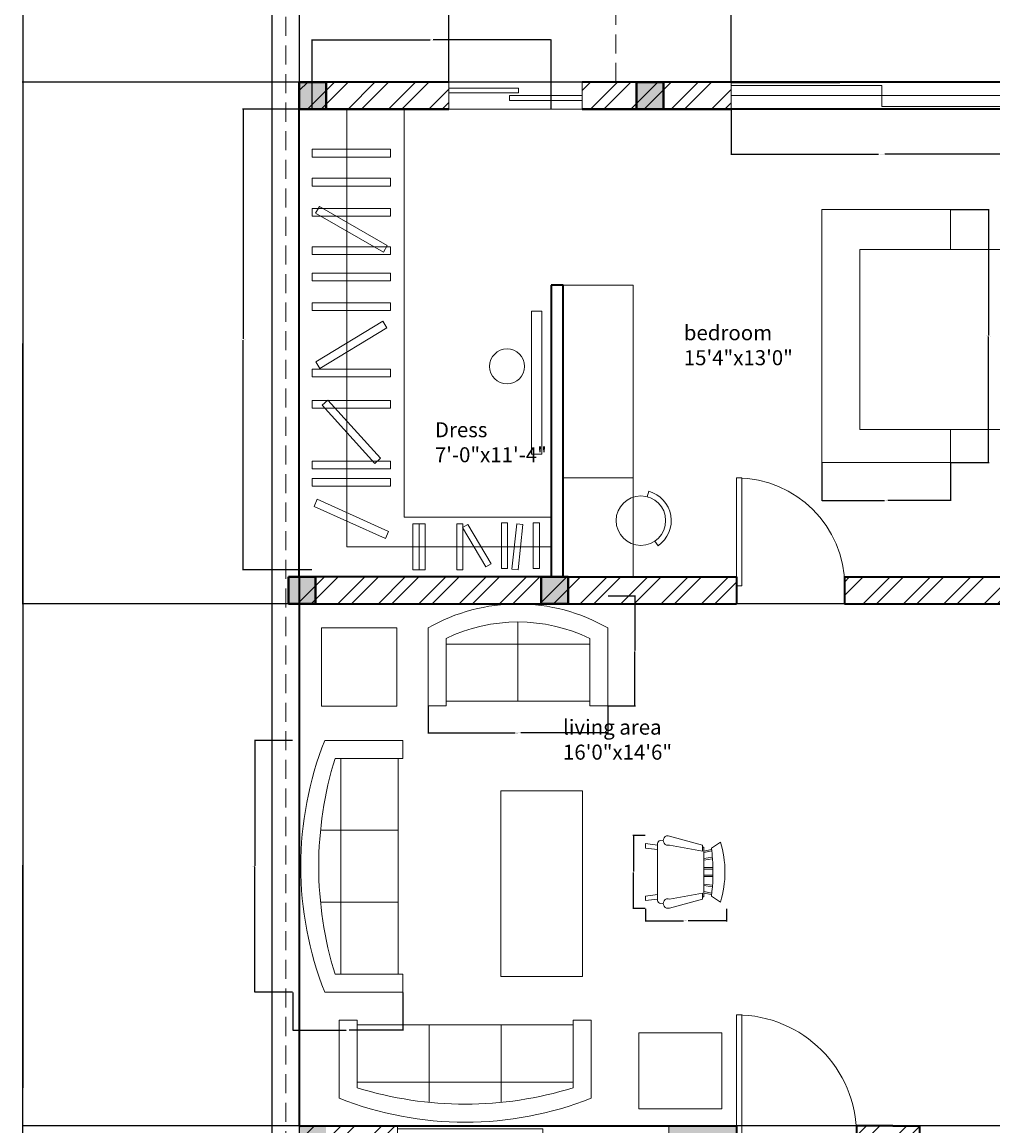
# Model space of a CAD drawing. Units: inches. Extents: x 19613 to 21413, y 12082 to 13202.
# Tile 3 of 9: x 19613 to 19937, y 12634 to 13002. Entities that reach past the tile are written whole.
import ezdxf

# ---------------------------------------------------------------- set-up
doc = ezdxf.new("R2010")
doc.units = ezdxf.units.IN
doc.linetypes.add('HIDDEN', pattern=[9.525, 6.35, -3.175])
for name, color, linetype, lineweight in [('A-ANNO-DIMS', 2, 'Continuous', 18), ('A-AREA-IDEN', 7, 'Continuous', 18), ('A-COLS', 7, 'Continuous', 40), ('A-COLS-PATT', 6, 'Continuous', 13), ('A-DOOR', 3, 'Continuous', 18), ('A-FLOR-CASE', 9, 'Continuous', 18), ('A-FLOR-HIDN', 8, 'HIDDEN', 13), ('A-FURN', 8, 'Continuous', 18), ('A-GLAZ', 4, 'Continuous', 18), ('A-WALL', 7, 'Continuous', 35), ('A-WALL-PATT', 252, 'Continuous', 13), ('C-PROP', 7, 'Continuous', 25), ('C-PROP-HIDN', 8, 'HIDDEN', 13)]:
    doc.layers.add(name, color=color, linetype=linetype, lineweight=lineweight)
doc.styles.get("Standard").update_dxf_attribs({"font": 'arial.ttf'})
doc.dimstyles.get("Standard").update_dxf_attribs({"dimtxt": 0.18, "dimasz": 0.18, "dimexe": 0.18, "dimexo": 0.0625, "dimgap": 0.09, "dimtad": 0, "dimtih": 1, "dimtoh": 1, "dimdec": 4, "dimzin": 0, "dimdsep": 46, "dimtxsty": 'Standard', "dimcen": 0.09, "dimadec": 0, "dimazin": 0, "dimtfac": 1, "dimtdec": 4, "dimtofl": 0, "dimtmove": 0, "dimatfit": 3, "dimfxl": 1, "dimtolj": 1, "dimtzin": 0, "dimarcsym": 0})

# ---------------------------------------------------------------- blocks, each defined once
blk = doc.blocks.new('*U4')
for p, q in [((0, 0), (0, -6)), ((36, 0), (36, -6))]:
    blk.add_line(p, q)
blk.add_lwpolyline([(0, 0), (0, 36), (1.75, 36), (1.75, 0)], close=True)
blk.add_arc((0, 0), 36, 0, 90)
blk = doc.blocks.new('Bed - Queen')
for p, q in [((0, -80.00003), (0, 0)), ((0, 0), (59.99999, 0)), ((59.99999, 0), (59.99999, -80.00003)), ((7.99999, -1.2), (28.79998, -1.2)), ((7.99999, -14.4), (7.99999, -1.2)), ((28.79998, -1.2), (28.79998, -14.4)), ((31.19999, -1.2), (51.99999, -1.2)), ((31.19999, -14.4), (31.19999, -1.2)), ((51.99999, -1.2), (51.99999, -16.4)), ((0, -14.4), (44.8, -14.4)), ((59.99999, -29.6), (44.8, -14.4)), ((44.8, -14.4), (44.8, -29.6)), ((44.8, -16.8), (0, -16.8)), ((51.99999, -16.4), (46.79936, -16.4)), ((44.8, -29.6), (59.99999, -29.6)), ((59.99999, -80.00003), (0, -80.00003))]:
    blk.add_line(p, q)
blk = doc.blocks.new('*U6')
for p, q in [((0, 0), (0, -6)), ((40, 0), (40, -6))]:
    blk.add_line(p, q)
blk.add_lwpolyline([(0, 0), (0, 40), (1.75, 40), (1.75, 0)], close=True)
blk.add_arc((0, 0), 40, 0, 90)
blk = doc.blocks.new('Sofa - Roundback Loveseat 5 ft.')
for p, q in [((0, -32.44198), (0, -5.99998)), ((-24, -33.99998), (-24, -11.46958)), ((-23.9998, -13.38178), (23.99986, -13.38178)), ((24.00004, -33.99998), (24.00004, -11.46958)), ((-24, -32.44198), (24.00004, -32.44198))]:
    blk.add_line(p, q)
for points in [[(-24, -33.99998), (-30, -33.99998), (-30, -7.99998)], [(30.00004, -7.99998), (30.00004, -33.99998), (24.00004, -33.99998)]]:
    blk.add_lwpolyline(points)
for centre, radius, start, end in [((0, -60.24998), 60.24998, 60.13715, 119.8628), ((0, -61.38438), 55.38444, 64.32083, 115.6792)]:
    blk.add_arc(centre, radius, start, end)
blk = doc.blocks.new('Sofa - Roundback 7 ft.')
for p, q in [((-12.00002, -32.4421), (-12.00003, -6.5971)), ((11.99997, -32.4421), (11.99998, -6.5971)), ((-36.000027, -34), (-36.000027, -11.4696)), ((-35.999844, -13.3819), (35.9998, -13.3819)), ((35.99998, -34), (35.99998, -11.4696)), ((-36.000027, -32.4421), (35.99998, -32.4421))]:
    blk.add_line(p, q)
for points in [[(-36.000027, -34), (-42.000027, -34), (-42.000027, -8)], [(41.99998, -8), (41.99998, -34), (35.99998, -34)]]:
    blk.add_lwpolyline(points)
for centre, radius, start, end in [((0, -114.25), 114.25, 68.43141, 111.5686), ((-0.00001, -127.1968), 121.1968, 72.72033, 107.2797)]:
    blk.add_arc(centre, radius, start, end)
blk = doc.blocks.new('Chair - Rocking')
for p, q in [((-8, -4.5), (-10, -1.5)), ((8, -4.5), (10, -1.5)), ((-8.23428, -6.99939), (-8.3093, -7.47958)), ((-8.23041, -7), (8.23915, -7)), ((-7.5, -4.5), (-7, -7)), ((-6.5, -7), (-7.02225, -4.43)), ((-4.5, -7), (-4.96674, -4.19951)), ((-4, -7), (-4.40532, -4.16272)), ((-1.5, -4.05012), (-1.5, -7)), ((-1, -7), (-1, -4.05012)), ((1, -7), (1, -4.04655)), ((1.5, -4.05012), (1.5, -7)), ((4, -7), (4.40187, -4.18694)), ((4.5, -7), (4.96761, -4.19437)), ((6.5, -7), (7, -4.4057)), ((7.5, -4.5), (7, -7)), ((8.31071, -7.48854), (8.23449, -7.00073)), ((-9, -7.5), (-12, -18.49999)), ((-7, -7.5), (-9, -7.5)), ((-9, -18.49999), (-7, -7.5)), ((7, -7.5), (9, -7.5)), ((9, -18.49999), (7, -7.5)), ((9, -7.5), (12, -18.49999)), ((-10.36644, -20.64523), (-10.5, -21.49999)), ((10.5, -21.49999), (10.3575, -20.58798)), ((-9, -22.49999), (-9.5, -26.49999)), ((0, -22.49999), (-9.5, -22.49999)), ((-8, -26.49999), (-7.5, -22.49999)), ((0, -22.49999), (9.5, -22.49999)), ((8, -26.49999), (7.5, -22.49999)), ((9, -22.49999), (9.5, -26.49999)), ((-9.5, -26.49999), (-8, -26.49999)), ((9.5, -26.49999), (8, -26.49999))]:
    blk.add_line(p, q)
for centre, radius, start, end in [((0, -34.08333), 34.08333, 72.93847, 107.0615), ((0, -68.25004), 64.25, 93.92211, 97.15267), ((0, -68.25004), 64.25, 82.84733, 93.92211), ((-10.5, -18.99999), 1.58114, 161.5651, 18.43495), ((-9.5, -21.49999), 1, 180, 270), ((10.5, -18.99999), 1.58114, 161.5651, 18.43495), ((9.5, -21.49999), 1, 270, 0)]:
    blk.add_arc(centre, radius, start, end)
blk = doc.blocks.new('COL-9x9')
for p, q in [((0, 9), (9, 9)), ((0, 0), (0, 9)), ((9, 9), (9, 0)), ((9, 0), (0, 0))]:
    blk.add_line(p, q)
blk = doc.blocks.new('CLOSET-L-RAIL')
for p, q in [((11.57, 153.64), (11.57, 7.7)), ((30.65, 153.64), (30.65, 17.54)), ((30.65, 17.54), (79.7, 17.54)), ((11.57, 7.7), (79.7, 7.7))]:
    blk.add_line(p, q)
for points in [[(0, 140.24), (26.12, 140.24), (26.12, 137.64), (0, 137.64)], [(0, 130.54), (26.12, 130.54), (26.12, 127.95), (0, 127.95)], [(0, 120.52), (26.12, 120.52), (26.12, 117.92), (0, 117.92)], [(2.39, 121.15), (25.03, 108.13), (23.74, 105.88), (1.09, 118.9)], [(0, 107.73), (26.12, 107.73), (26.12, 105.13), (0, 105.13)], [(0, 98.91), (26.12, 98.91), (26.12, 96.32), (0, 96.32)], [(0, 89.07), (26.12, 89.07), (26.12, 86.48), (0, 86.48)], [(1.22, 69.39), (23.56, 82.95), (24.9, 80.73), (2.57, 67.18)], [(0, 66.96), (26.12, 66.96), (26.12, 64.37), (0, 64.37)], [(0, 56.45), (26.12, 56.45), (26.12, 53.86), (0, 53.86)], [(5.27, 56.6), (22.78, 37.21), (20.85, 35.47), (3.35, 54.86)], [(0, 36.27), (26.12, 36.27), (26.12, 33.68), (0, 33.68)], [(0, 30.47), (26.12, 30.47), (26.12, 27.88), (0, 27.88)], [(1.67, 23.53), (25.51, 12.85), (24.45, 10.49), (0.61, 21.17)], [(35.67, 0.07), (33.61, 0.07), (33.61, 15.33), (35.67, 15.33)], [(37.73, 0.07), (35.67, 0.07), (35.67, 15.33), (37.73, 15.33)], [(50.3, 0.07), (48.24, 0.07), (48.24, 15.33), (50.3, 15.33)], [(59.69, 2.02), (57.92, 0.97), (50.13, 14.1), (51.9, 15.15)], [(65.15, 0.43), (63.09, 0.43), (63.09, 15.69), (65.15, 15.69)], [(68.26, 15.4), (70.31, 15.18), (68.65, 0), (66.6, 0.22)], [(75.77, 0.43), (73.71, 0.43), (73.71, 15.69), (75.77, 15.69)]]:
    blk.add_lwpolyline(points, close=True)
blk = doc.blocks.new('WINDOW-LIVING-SLIDER')
for p, q in [((0, 9), (0, 0)), ((0, 8.08), (48.53, 8.08)), ((48.53, 4.5), (48.53, 8.08)), ((48.53, 8.08), (48.53, 1.28)), ((90.49, 9), (90.49, 0)), ((0, 4.5), (48.53, 4.5)), ((48.53, 1.28), (48.53, 4.5)), ((48.53, 4.5), (90.49, 4.5)), ((90.49, 6.86), (90.49, 4.5)), ((48.53, 1.28), (90.49, 1.28))]:
    blk.add_line(p, q)
blk = doc.blocks.new('WINDOW-BEDROOM-SLIDER')
for p, q in [((0, 9), (0, 0)), ((0, 9), (100.32, 9)), ((0, 0), (0, 9)), ((50.28, 7.85), (0, 7.85)), ((50.28, 4.5), (50.28, 7.85)), ((50.28, 7.85), (50.28, 4.5)), ((100.32, 9), (100.32, 0)), ((100.32, 9), (100.32, 0.84)), ((0, 4.5), (50.28, 4.5)), ((50.28, 4.5), (100.32, 4.5)), ((100.32, 4.5), (50.28, 4.5)), ((50.28, 4.5), (50.28, 0.84)), ((50.28, 0.84), (100.32, 0.84)), ((100.32, 0.84), (100.32, 0)), ((100.32, 0), (0, 0))]:
    blk.add_line(p, q)
blk = doc.blocks.new('WINDOW-DRESS-SLIDER')
for p, q in [((0, 9), (0, 0)), ((0, 9), (44.45, 9)), ((44.45, 9), (44.45, 0)), ((0, 0), (44.45, 0))]:
    blk.add_line(p, q)
for points in [[(0, 6.95), (23.27, 6.95), (23.27, 5.37), (0, 5.37)], [(44.45, 4.5), (20.22, 4.5), (20.22, 2.83), (44.45, 2.83)]]:
    blk.add_lwpolyline(points, close=True)
blk = doc.blocks.new('DESK-CHAIR-ROUND')
for p, q in [((10.85, 18.16), (10.37, 16.34)), ((13.96, 0), (12.89, 1.56))]:
    blk.add_line(p, q)
blk.add_circle((8.25, 8.37), 8.25)
blk.add_arc((8.25, 8.37), 10.13, 304.3105, 75.0908)
blk = doc.blocks.new('BEDROOM-DESK-SLIM')
for p, q in [((0, 97.32), (23.4, 97.32)), ((23.4, 97.32), (23.4, 0)), ((0, 33.03), (23.4, 33.03))]:
    blk.add_line(p, q)
blk = doc.blocks.new('BEDROOM-AREA-RUG')
for p, q in [((42.96, 84.39), (0, 84.39)), ((0, 84.39), (0, 0)), ((42.96, 71.03), (42.96, 84.39)), ((12.72, 71.03), (42.96, 71.03)), ((42.96, 0), (42.96, 11.03)), ((0, 0), (42.96, 0))]:
    blk.add_line(p, q)
blk = doc.blocks.new('*D49')
at = {"layer": 'A-ANNO-DIMS', "color": 0, "lineweight": -2, "transparency": 16777216}
for p, q in [((19703.45, 12762.82), (19690.73, 12762.82)), ((19690.91, 12762.64), (19690.91, 12721)), ((19690.91, 12679), (19690.91, 12720.64)), ((19703.45, 12678.82), (19690.73, 12678.82))]:
    blk.add_line(p, q, dxfattribs=at)
at = {"layer": 'A-ANNO-DIMS', "color": 0, "transparency": 16777216}
for points in [[(19690.88, 12762.64), (19690.94, 12762.64), (19690.91, 12762.82)], [(19690.88, 12679), (19690.94, 12679), (19690.91, 12678.82)]]:
    blk.add_solid(points, dxfattribs=at)
at = {"layer": 'Defpoints', "color": 0, "transparency": 16777216}
for p in [(19690.91, 12762.82), (19703.51, 12762.82), (19703.51, 12678.82)]:
    blk.add_point(p, dxfattribs=at)
at = {"layer": 'A-ANNO-DIMS', "color": 0, "transparency": 16777216, "insert": (19690.91, 12720.82), "char_height": 0.18, "attachment_point": 5}
blk.add_mtext('\\A1;SOFA 84 TYP.', dxfattribs=at)
blk = doc.blocks.new('*D50')
at = {"layer": 'A-ANNO-DIMS', "color": 0, "lineweight": -2, "transparency": 16777216}
for p, q in [((19703.51, 12678.76), (19703.51, 12666.04)), ((19740.18, 12678.76), (19740.18, 12666.04)), ((19703.69, 12666.22), (19721.32, 12666.22)), ((19740, 12666.22), (19722.37, 12666.22))]:
    blk.add_line(p, q, dxfattribs=at)
at = {"layer": 'A-ANNO-DIMS', "color": 0, "transparency": 16777216}
for points in [[(19703.69, 12666.25), (19703.69, 12666.19), (19703.51, 12666.22)], [(19740, 12666.25), (19740, 12666.19), (19740.18, 12666.22)]]:
    blk.add_solid(points, dxfattribs=at)
at = {"layer": 'Defpoints', "color": 0, "transparency": 16777216}
for p in [(19703.51, 12678.82), (19740.18, 12678.82), (19703.51, 12666.22)]:
    blk.add_point(p, dxfattribs=at)
at = {"layer": 'A-ANNO-DIMS', "color": 0, "transparency": 16777216, "insert": (19721.85, 12666.22), "char_height": 0.18, "attachment_point": 5}
blk.add_mtext('\\A1;37 TYP.', dxfattribs=at)
blk = doc.blocks.new('*D55')
at = {"layer": 'A-ANNO-DIMS', "color": 0, "lineweight": -2, "transparency": 16777216}
for p, q in [((19709.93, 12973.28), (19686.76, 12973.28)), ((19686.94, 12973.1), (19686.94, 12896.64)), ((19686.94, 12819.82), (19686.94, 12896.28)), ((19709.93, 12819.64), (19686.76, 12819.64))]:
    blk.add_line(p, q, dxfattribs=at)
at = {"layer": 'A-ANNO-DIMS', "color": 0, "transparency": 16777216}
for points in [[(19686.91, 12973.1), (19686.97, 12973.1), (19686.94, 12973.28)], [(19686.91, 12819.82), (19686.97, 12819.82), (19686.94, 12819.64)]]:
    blk.add_solid(points, dxfattribs=at)
at = {"layer": 'Defpoints', "color": 0, "transparency": 16777216}
for p in [(19686.94, 12973.28), (19709.99, 12973.28), (19709.99, 12819.64)]:
    blk.add_point(p, dxfattribs=at)
at = {"layer": 'A-ANNO-DIMS', "color": 0, "transparency": 16777216, "insert": (19686.94, 12896.46), "char_height": 0.18, "attachment_point": 5}
blk.add_mtext('\\A1;L-RAIL 154 TYP.', dxfattribs=at)
blk = doc.blocks.new('*D56')
at = {"layer": 'A-ANNO-DIMS', "color": 0, "lineweight": -2, "transparency": 16777216}
for p, q in [((19709.99, 12973.34), (19709.99, 12996.5)), ((19710.17, 12996.32), (19749.31, 12996.32)), ((19789.51, 12996.32), (19750.37, 12996.32)), ((19789.69, 12973.34), (19789.69, 12996.5))]:
    blk.add_line(p, q, dxfattribs=at)
at = {"layer": 'A-ANNO-DIMS', "color": 0, "transparency": 16777216}
for points in [[(19710.17, 12996.35), (19710.17, 12996.29), (19709.99, 12996.32)], [(19789.51, 12996.35), (19789.51, 12996.29), (19789.69, 12996.32)]]:
    blk.add_solid(points, dxfattribs=at)
at = {"layer": 'Defpoints', "color": 0, "transparency": 16777216}
for p in [(19789.69, 12996.32), (19709.99, 12973.28), (19789.69, 12973.28)]:
    blk.add_point(p, dxfattribs=at)
at = {"layer": 'A-ANNO-DIMS', "color": 0, "transparency": 16777216, "insert": (19749.84, 12996.32), "char_height": 0.18, "attachment_point": 5}
blk.add_mtext('\\A1;80 TYP.', dxfattribs=at)
blk = doc.blocks.new('*D61')
at = {"layer": 'A-ANNO-DIMS', "color": 0, "lineweight": -2, "transparency": 16777216}
for p, q in [((19849.73, 12973.22), (19849.73, 12958.05)), ((19950.05, 12973.22), (19950.05, 12958.05)), ((19849.91, 12958.23), (19898.81, 12958.23)), ((19949.87, 12958.23), (19900.98, 12958.23))]:
    blk.add_line(p, q, dxfattribs=at)
at = {"layer": 'A-ANNO-DIMS', "color": 0, "transparency": 16777216}
for points in [[(19849.91, 12958.26), (19849.91, 12958.2), (19849.73, 12958.23)], [(19949.87, 12958.26), (19949.87, 12958.2), (19950.05, 12958.23)]]:
    blk.add_solid(points, dxfattribs=at)
at = {"layer": 'Defpoints', "color": 0, "transparency": 16777216}
for p in [(19849.73, 12973.28), (19950.05, 12973.28), (19950.05, 12958.23)]:
    blk.add_point(p, dxfattribs=at)
at = {"layer": 'A-ANNO-DIMS', "color": 0, "transparency": 16777216, "insert": (19899.89, 12958.23), "char_height": 0.18, "attachment_point": 5}
blk.add_mtext('\\A1;SLIDER 100 TYP.', dxfattribs=at)
blk = doc.blocks.new('*D75')
at = {"layer": 'A-ANNO-DIMS', "color": 0, "lineweight": -2, "transparency": 16777216}
for p, q in [((19922.95, 12939.84), (19935.73, 12939.84)), ((19935.55, 12939.66), (19935.55, 12897.83)), ((19935.55, 12855.63), (19935.55, 12897.46)), ((19922.95, 12855.45), (19935.73, 12855.45))]:
    blk.add_line(p, q, dxfattribs=at)
at = {"layer": 'A-ANNO-DIMS', "color": 0, "transparency": 16777216}
for points in [[(19935.52, 12939.66), (19935.58, 12939.66), (19935.55, 12939.84)], [(19935.52, 12855.63), (19935.58, 12855.63), (19935.55, 12855.45)]]:
    blk.add_solid(points, dxfattribs=at)
at = {"layer": 'Defpoints', "color": 0, "transparency": 16777216}
for p in [(19922.89, 12939.84), (19935.55, 12939.84), (19922.89, 12855.45)]:
    blk.add_point(p, dxfattribs=at)
at = {"layer": 'A-ANNO-DIMS', "color": 0, "transparency": 16777216, "insert": (19935.55, 12897.65), "char_height": 0.18, "attachment_point": 5}
blk.add_mtext('\\A1;RUG 84 TYP.', dxfattribs=at)
blk = doc.blocks.new('*D76')
at = {"layer": 'A-ANNO-DIMS', "color": 0, "lineweight": -2, "transparency": 16777216}
for p, q in [((19879.93, 12855.39), (19879.93, 12842.61)), ((19922.89, 12855.39), (19922.89, 12842.61)), ((19880.11, 12842.79), (19900.88, 12842.79)), ((19922.71, 12842.79), (19901.94, 12842.79))]:
    blk.add_line(p, q, dxfattribs=at)
at = {"layer": 'A-ANNO-DIMS', "color": 0, "transparency": 16777216}
for points in [[(19880.11, 12842.82), (19880.11, 12842.76), (19879.93, 12842.79)], [(19922.71, 12842.82), (19922.71, 12842.76), (19922.89, 12842.79)]]:
    blk.add_solid(points, dxfattribs=at)
at = {"layer": 'Defpoints', "color": 0, "transparency": 16777216}
for p in [(19879.93, 12855.45), (19922.89, 12855.45), (19922.89, 12842.79)]:
    blk.add_point(p, dxfattribs=at)
at = {"layer": 'A-ANNO-DIMS', "color": 0, "transparency": 16777216, "insert": (19901.41, 12842.79), "char_height": 0.18, "attachment_point": 5}
blk.add_mtext('\\A1;43 TYP.', dxfattribs=at)
blk = doc.blocks.new('*D79')
at = {"layer": 'A-ANNO-DIMS', "color": 0, "lineweight": -2, "transparency": 16777216}
for p, q in [((19748.62, 12774.22), (19748.62, 12765.1)), ((19808.62, 12774.22), (19808.62, 12765.1)), ((19748.8, 12765.28), (19777.71, 12765.28)), ((19808.44, 12765.28), (19779.54, 12765.28))]:
    blk.add_line(p, q, dxfattribs=at)
at = {"layer": 'A-ANNO-DIMS', "color": 0, "transparency": 16777216}
for points in [[(19748.8, 12765.31), (19748.8, 12765.25), (19748.62, 12765.28)], [(19808.44, 12765.31), (19808.44, 12765.25), (19808.62, 12765.28)]]:
    blk.add_solid(points, dxfattribs=at)
at = {"layer": 'Defpoints', "color": 0, "transparency": 16777216}
for p in [(19748.62, 12774.28), (19808.62, 12774.28), (19808.62, 12765.28)]:
    blk.add_point(p, dxfattribs=at)
at = {"layer": 'A-ANNO-DIMS', "color": 0, "transparency": 16777216, "insert": (19778.62, 12765.28), "char_height": 0.18, "attachment_point": 5}
blk.add_mtext('\\A1;LOVESEAT 60', dxfattribs=at)
blk = doc.blocks.new('*D80')
at = {"layer": 'A-ANNO-DIMS', "color": 0, "lineweight": -2, "transparency": 16777216}
for p, q in [((19808.68, 12810.95), (19817.8, 12810.95)), ((19817.62, 12810.77), (19817.62, 12792.79)), ((19817.62, 12774.46), (19817.62, 12792.43)), ((19808.68, 12774.28), (19817.8, 12774.28))]:
    blk.add_line(p, q, dxfattribs=at)
at = {"layer": 'A-ANNO-DIMS', "color": 0, "transparency": 16777216}
for points in [[(19817.59, 12810.77), (19817.65, 12810.77), (19817.62, 12810.95)], [(19817.59, 12774.46), (19817.65, 12774.46), (19817.62, 12774.28)]]:
    blk.add_solid(points, dxfattribs=at)
at = {"layer": 'Defpoints', "color": 0, "transparency": 16777216}
for p in [(19808.62, 12810.95), (19817.62, 12810.95), (19808.62, 12774.28)]:
    blk.add_point(p, dxfattribs=at)
at = {"layer": 'A-ANNO-DIMS', "color": 0, "transparency": 16777216, "insert": (19817.62, 12792.61), "char_height": 0.18, "attachment_point": 5}
blk.add_mtext('\\A1;37', dxfattribs=at)
blk = doc.blocks.new('*D81')
at = {"layer": 'A-ANNO-DIMS', "color": 0, "lineweight": -2, "transparency": 16777216}
for p, q in [((19821.16, 12706.65), (19821.16, 12702.48)), ((19848.16, 12706.65), (19848.16, 12702.48)), ((19821.34, 12702.66), (19833.87, 12702.66)), ((19847.98, 12702.66), (19835.44, 12702.66))]:
    blk.add_line(p, q, dxfattribs=at)
at = {"layer": 'A-ANNO-DIMS', "color": 0, "transparency": 16777216}
for points in [[(19821.34, 12702.69), (19821.34, 12702.63), (19821.16, 12702.66)], [(19847.98, 12702.69), (19847.98, 12702.63), (19848.16, 12702.66)]]:
    blk.add_solid(points, dxfattribs=at)
at = {"layer": 'Defpoints', "color": 0, "transparency": 16777216}
for p in [(19821.16, 12706.71), (19848.16, 12706.71), (19848.16, 12702.66)]:
    blk.add_point(p, dxfattribs=at)
at = {"layer": 'A-ANNO-DIMS', "color": 0, "transparency": 16777216, "insert": (19834.66, 12702.66), "char_height": 0.18, "attachment_point": 5}
blk.add_mtext('\\A1;ROCKER 27', dxfattribs=at)
blk = doc.blocks.new('*D82')
at = {"layer": 'A-ANNO-DIMS', "color": 0, "lineweight": -2, "transparency": 16777216}
for p, q in [((19821.09, 12731.14), (19816.93, 12731.14)), ((19817.11, 12730.96), (19817.11, 12719.11)), ((19817.11, 12706.89), (19817.11, 12718.75)), ((19821.09, 12706.71), (19816.93, 12706.71))]:
    blk.add_line(p, q, dxfattribs=at)
at = {"layer": 'A-ANNO-DIMS', "color": 0, "transparency": 16777216}
for points in [[(19817.08, 12730.96), (19817.14, 12730.96), (19817.11, 12731.14)], [(19817.08, 12706.89), (19817.14, 12706.89), (19817.11, 12706.71)]]:
    blk.add_solid(points, dxfattribs=at)
at = {"layer": 'Defpoints', "color": 0, "transparency": 16777216}
for p in [(19821.16, 12731.14), (19817.11, 12706.71), (19821.16, 12706.71)]:
    blk.add_point(p, dxfattribs=at)
at = {"layer": 'A-ANNO-DIMS', "color": 0, "transparency": 16777216, "insert": (19817.11, 12718.93), "char_height": 0.18, "attachment_point": 5}
blk.add_mtext('\\A1;24', dxfattribs=at)
blk = doc.blocks.new('*D84')
at = {"layer": 'A-ANNO-DIMS', "color": 0, "lineweight": -2, "transparency": 16777216}
for p, q in [((19696.63, 13118.28), (19613.26, 13118.28)), ((19613.44, 13118.1), (19613.44, 12646.96)), ((19613.44, 12175.46), (19613.44, 12646.6)), ((19696.63, 12175.28), (19613.26, 12175.28))]:
    blk.add_line(p, q, dxfattribs=at)
at = {"layer": 'A-ANNO-DIMS', "color": 0, "transparency": 16777216}
for points in [[(19613.41, 13118.1), (19613.47, 13118.1), (19613.44, 13118.28)], [(19613.41, 12175.46), (19613.47, 12175.46), (19613.44, 12175.28)]]:
    blk.add_solid(points, dxfattribs=at)
at = {"layer": 'Defpoints', "color": 0, "transparency": 16777216}
for p in [(19613.44, 13118.28), (19696.69, 13118.28), (19696.69, 12175.28)]:
    blk.add_point(p, dxfattribs=at)
at = {"layer": 'A-ANNO-DIMS', "color": 0, "transparency": 16777216, "insert": (19613.44, 12646.78), "char_height": 0.18, "attachment_point": 5}
blk.add_mtext('\\A1;943', dxfattribs=at)
blk = doc.blocks.new('*D89')
at = {"layer": 'A-ANNO-DIMS', "color": 0, "lineweight": -2, "transparency": 16777216}
for p, q in [((20807.37, 12808.28), (19613.26, 12808.28)), ((19613.44, 12808.1), (19613.44, 12721.46)), ((19613.44, 12634.46), (19613.44, 12721.1)), ((20807.37, 12634.28), (19613.26, 12634.28))]:
    blk.add_line(p, q, dxfattribs=at)
at = {"layer": 'A-ANNO-DIMS', "color": 0, "transparency": 16777216}
for points in [[(19613.41, 12808.1), (19613.47, 12808.1), (19613.44, 12808.28)], [(19613.41, 12634.46), (19613.47, 12634.46), (19613.44, 12634.28)]]:
    blk.add_solid(points, dxfattribs=at)
at = {"layer": 'Defpoints', "color": 0, "transparency": 16777216}
for p in [(19613.44, 12808.28), (20807.43, 12808.28), (20807.43, 12634.28)]:
    blk.add_point(p, dxfattribs=at)
at = {"layer": 'A-ANNO-DIMS', "color": 0, "transparency": 16777216, "insert": (19613.44, 12721.28), "char_height": 0.18, "attachment_point": 5}
blk.add_mtext('\\A1;174', dxfattribs=at)
blk = doc.blocks.new('*D90')
at = {"layer": 'A-ANNO-DIMS', "color": 0, "lineweight": -2, "transparency": 16777216}
for p, q in [((20807.37, 12982.28), (19613.26, 12982.28)), ((19613.44, 12982.1), (19613.44, 12895.46)), ((19613.44, 12808.46), (19613.44, 12895.1)), ((20807.37, 12808.28), (19613.26, 12808.28))]:
    blk.add_line(p, q, dxfattribs=at)
at = {"layer": 'A-ANNO-DIMS', "color": 0, "transparency": 16777216}
for points in [[(19613.41, 12982.1), (19613.47, 12982.1), (19613.44, 12982.28)], [(19613.41, 12808.46), (19613.47, 12808.46), (19613.44, 12808.28)]]:
    blk.add_solid(points, dxfattribs=at)
at = {"layer": 'Defpoints', "color": 0, "transparency": 16777216}
for p in [(19613.44, 12982.28), (20807.43, 12982.28), (20807.43, 12808.28)]:
    blk.add_point(p, dxfattribs=at)
at = {"layer": 'A-ANNO-DIMS', "color": 0, "transparency": 16777216, "insert": (19613.44, 12895.28), "char_height": 0.18, "attachment_point": 5}
blk.add_mtext('\\A1;174', dxfattribs=at)
blk = doc.blocks.new('*D101')
at = {"layer": 'A-ANNO-DIMS', "color": 0, "lineweight": -2, "transparency": 16777216}
for p, q in [((19755.54, 12982.34), (19755.54, 13201.71)), ((19755.72, 13201.53), (19802.31, 13201.53)), ((19849.55, 13201.53), (19802.96, 13201.53)), ((19849.73, 12982.34), (19849.73, 13201.71))]:
    blk.add_line(p, q, dxfattribs=at)
at = {"layer": 'A-ANNO-DIMS', "color": 0, "transparency": 16777216}
for points in [[(19755.72, 13201.56), (19755.72, 13201.5), (19755.54, 13201.53)], [(19849.55, 13201.56), (19849.55, 13201.5), (19849.73, 13201.53)]]:
    blk.add_solid(points, dxfattribs=at)
at = {"layer": 'Defpoints', "color": 0, "transparency": 16777216}
for p in [(19849.73, 13201.53), (19755.54, 12982.28), (19849.73, 12982.28)]:
    blk.add_point(p, dxfattribs=at)
at = {"layer": 'A-ANNO-DIMS', "color": 0, "transparency": 16777216, "insert": (19802.63, 13201.53), "char_height": 0.18, "attachment_point": 5}
blk.add_mtext('\\A1;94.2', dxfattribs=at)
blk = doc.blocks.new('*D102')
at = {"layer": 'A-ANNO-DIMS', "color": 0, "lineweight": -2, "transparency": 16777216}
for p, q in [((19849.73, 12982.34), (19849.73, 13201.71)), ((19849.91, 13201.53), (19924.46, 13201.53)), ((19999.93, 13201.53), (19925.37, 13201.53)), ((20000.11, 12982.34), (20000.11, 13201.71))]:
    blk.add_line(p, q, dxfattribs=at)
at = {"layer": 'A-ANNO-DIMS', "color": 0, "transparency": 16777216}
for points in [[(19849.91, 13201.56), (19849.91, 13201.5), (19849.73, 13201.53)], [(19999.93, 13201.56), (19999.93, 13201.5), (20000.11, 13201.53)]]:
    blk.add_solid(points, dxfattribs=at)
at = {"layer": 'Defpoints', "color": 0, "transparency": 16777216}
for p in [(20000.11, 13201.53), (19849.73, 12982.28), (20000.11, 12982.28)]:
    blk.add_point(p, dxfattribs=at)
at = {"layer": 'A-ANNO-DIMS', "color": 0, "transparency": 16777216, "insert": (19924.92, 13201.53), "char_height": 0.18, "attachment_point": 5}
blk.add_mtext('\\A1;150.37', dxfattribs=at)

msp = doc.modelspace()

# ---------------------------------------------------------------- hatches: boundary and pattern name
at = {"layer": 'A-COLS-PATT'}
h = msp.add_hatch(color=256, dxfattribs=at)
h.dxf.hatch_style = 1
h.paths.add_polyline_path([(19701.1937, 13118.279), (19696.6937, 13118.279), (19696.6937, 13113.779), (19701.1937, 13113.779)])
h.paths.add_polyline_path([(19714.6694, 12982.279), (19705.6937, 12982.279), (19705.6937, 12973.279), (19714.6694, 12973.279)])
h.paths.add_polyline_path([(19827.1183, 12982.279), (19818.1183, 12982.279), (19818.1183, 12973.279), (19827.1183, 12973.279)])
h.paths.add_polyline_path([(19982.6937, 12982.279), (19973.6937, 12982.279), (19973.6937, 12973.279), (19982.6937, 12973.279)])
h.paths.add_polyline_path([(19982.6937, 12817.279), (19973.6937, 12817.279), (19973.6937, 12808.279), (19982.6937, 12808.279)])
h.paths.add_polyline_path([(19795.361, 12817.279), (19786.361, 12817.279), (19786.361, 12808.279), (19795.361, 12808.279)])
h.paths.add_polyline_path([(19705.6937, 12817.279), (19702.0819, 12817.279), (19702.0819, 12808.279), (19705.6937, 12808.279)])
h.paths.add_polyline_path([(19711.0819, 12817.279), (19705.6937, 12817.279), (19705.6937, 12808.279), (19711.0819, 12808.279)])
h.paths.add_polyline_path([(19714.6136, 12634.279), (19705.6937, 12634.279), (19705.6937, 12625.279), (19714.6136, 12625.279)])
h.paths.add_polyline_path([(19705.6937, 12485.8897), (19701.1937, 12485.8897), (19701.1937, 12476.8897), (19705.6937, 12476.8897)])
h.paths.add_polyline_path([(19709.3479, 12485.8897), (19705.6937, 12485.8897), (19705.6937, 12476.8897), (19709.3479, 12476.8897)])
h.paths.add_polyline_path([(19701.1937, 12485.8897), (19700.3479, 12485.8897), (19700.3479, 12476.8897), (19701.1937, 12476.8897)])
h.paths.add_polyline_path([(20218.6937, 12421.279), (20209.6937, 12421.279), (20209.6937, 12412.279), (20218.6937, 12412.279)])
h.paths.add_polyline_path([(20218.6937, 12634.279), (20209.6937, 12634.279), (20209.6937, 12625.279), (20218.6937, 12625.279)])
h.paths.add_polyline_path([(20218.6937, 12808.279), (20209.6937, 12808.279), (20209.6937, 12803.279), (20218.6937, 12803.279)])
h.paths.add_polyline_path([(20218.6937, 12810.1878), (20209.6937, 12810.1878), (20209.6937, 12808.279), (20218.6937, 12808.279)])
h.paths.add_polyline_path([(20218.6937, 12803.279), (20209.6937, 12803.279), (20209.6937, 12801.1878), (20218.6937, 12801.1878)])
h.paths.add_polyline_path([(20218.6937, 12982.279), (20209.6937, 12982.279), (20209.6937, 12973.279), (20218.6937, 12973.279)])
h.paths.add_polyline_path([(20100.1214, 12982.279), (20080.8386, 12982.279), (20080.8386, 12973.279), (20091.6937, 12973.279), (20100.1214, 12973.279), (20100.1214, 12976.279)])
h.paths.add_polyline_path([(19851.5503, 12631.279), (19851.5503, 12634.279), (19828.8814, 12634.279), (19828.8814, 12625.279), (19851.5503, 12625.279)])
at = {"layer": 'A-WALL-PATT'}
h = msp.add_hatch(dxfattribs=at)
h.set_pattern_fill('ANSI32', color=256)
h.paths.add_polyline_path([(20223.1937, 13118.279), (20218.6937, 13118.279), (19701.1937, 13118.279), (19701.1937, 13113.779), (20223.1937, 13113.779)])
h.paths.add_polyline_path([(19849.7315, 12982.279), (19799.9854, 12982.279), (19799.9854, 12973.279), (19849.7315, 12973.279)])
h.paths.add_polyline_path([(19755.5378, 12982.279), (19705.6937, 12982.279), (19705.6937, 12973.279), (19755.5378, 12973.279)])
h.paths.add_polyline_path([(20000.1054, 12982.279), (19950.0534, 12982.279), (19950.0534, 12974.1171), (19950.0534, 12973.279), (20000.1054, 12973.279)])
h.paths.add_polyline_path([(20049.4797, 12982.279), (20030.7476, 12982.279), (20030.7476, 12973.279), (20049.4797, 12973.279)])
h.paths.add_polyline_path([(20100.1214, 12982.279), (20080.8386, 12982.279), (20080.8386, 12973.279), (20100.1214, 12973.279), (20100.1214, 12976.279)])
h.paths.add_polyline_path([(20218.6937, 12982.279), (20167.6937, 12982.279), (20140.1214, 12982.279), (20140.1214, 12976.279, -0.01769781), (20140.0212, 12973.45), (20167.6937, 12973.279), (20176.6937, 12973.279), (20218.6937, 12973.279)])
h.paths.add_polyline_path([(19851.5503, 12814.279), (19851.5503, 12817.279), (19793.6937, 12817.279), (19789.6937, 12817.279), (19705.6937, 12817.279), (19705.6937, 12808.279), (19851.5503, 12808.279)])
h.paths.add_polyline_path([(19982.6937, 12973.279), (19973.6937, 12973.279), (19973.6937, 12817.279), (19887.5503, 12817.279), (19887.5503, 12808.279), (19973.6937, 12808.279), (19982.6937, 12808.279)])
h.paths.add_polyline_path([(20058.6937, 12850.5529), (19982.6937, 12850.5529), (19982.6937, 12846.5529), (20058.6937, 12846.5529)])
h.paths.add_polyline_path([(20095.6937, 12973.279), (20091.6937, 12973.279), (20091.6937, 12850.5529), (20087.6937, 12850.5529), (20087.6937, 12846.5529), (20095.6937, 12846.5529)])
h.paths.add_polyline_path([(20218.6937, 12808.279), (20140.8605, 12808.279), (20126.9413, 12808.279), (20126.9413, 12803.279), (20140.8605, 12803.279), (20218.6937, 12803.279)])
h.paths.add_polyline_path([(19738.3931, 12634.279), (19705.6937, 12634.279), (19705.6937, 12625.279), (19738.3931, 12625.279)])
h.paths.add_polyline_path([(19912.6937, 12634.279), (19903.6937, 12634.279), (19891.5503, 12634.279), (19891.5503, 12625.279), (19903.6937, 12625.279), (19903.6937, 12445.279), (19975.6937, 12445.279), (20128.6937, 12445.279), (20128.6937, 12412.279), (20149.8479, 12412.279), (20149.8479, 12421.279), (20137.6937, 12421.279), (20137.6937, 12454.279), (20137.6937, 12580.2801), (20133.6937, 12580.2801), (20133.6937, 12454.279), (19984.6937, 12454.279), (19984.6937, 12625.279), (19993.6937, 12625.279), (19993.6937, 12634.279), (19984.6937, 12634.279), (19975.6937, 12634.279), (19975.6937, 12454.279), (19912.6937, 12454.279)])
h.paths.add_polyline_path([(20218.6937, 12634.279), (20137.6937, 12634.279), (20029.6937, 12634.279), (20029.6937, 12625.279), (20137.6937, 12625.279), (20218.6937, 12625.279)])
h.paths.add_polyline_path([(21014.4339, 12634.279), (21005.4339, 12634.279), (20993.2905, 12634.279), (20993.2905, 12625.279), (21005.4339, 12625.279), (21005.4339, 12445.279), (21077.4339, 12445.279), (21230.4339, 12445.279), (21230.4339, 12412.279), (21251.5881, 12412.279), (21251.5881, 12421.279), (21239.4339, 12421.279), (21239.4339, 12454.279), (21239.4339, 12580.2801), (21235.4339, 12580.2801), (21235.4339, 12454.279), (21086.4339, 12454.279), (21086.4339, 12625.279), (21095.4339, 12625.279), (21095.4339, 12634.279), (21086.4339, 12634.279), (21077.4339, 12634.279), (21077.4339, 12454.279), (21014.4339, 12454.279)])
h.paths.add_polyline_path([(20840.1333, 12634.279), (20807.4339, 12634.279), (20807.4339, 12625.279), (20840.1333, 12625.279)])
h.paths.add_polyline_path([(20953.2905, 12631.279), (20953.2905, 12634.279), (20930.6216, 12634.279), (20930.6216, 12625.279), (20953.2905, 12625.279)])
h.paths.add_polyline_path([(21320.4339, 12634.279), (21239.4339, 12634.279), (21131.4339, 12634.279), (21131.4339, 12625.279), (21239.4339, 12625.279), (21320.4339, 12625.279)])
h.paths.add_polyline_path([(21084.4339, 12973.279), (21075.4339, 12973.279), (21075.4339, 12817.279), (20989.2905, 12817.279), (20989.2905, 12808.279), (21075.4339, 12808.279), (21084.4339, 12808.279)])
h.paths.add_polyline_path([(21142.1261, 12863.2893), (21084.4339, 12863.2893), (21084.4339, 12846.5529), (21142.1261, 12846.5529)])
h.paths.add_polyline_path([(21320.4339, 12808.279), (21242.6007, 12808.279), (21228.6815, 12808.279), (21228.6815, 12803.279), (21242.6007, 12803.279), (21320.4339, 12803.279)])
h.paths.add_polyline_path([(20857.278, 12982.279), (20807.4339, 12982.279), (20807.4339, 12973.279), (20857.278, 12973.279)])
h.paths.add_polyline_path([(20951.4717, 12982.279), (20901.7255, 12982.279), (20901.7255, 12973.279), (20951.4717, 12973.279)])
h.paths.add_polyline_path([(21101.8455, 12982.279), (21051.7936, 12982.279), (21051.7936, 12974.1171), (21051.7936, 12973.279), (21101.8455, 12973.279)])
h.paths.add_polyline_path([(21151.2199, 12982.279), (21132.4878, 12982.279), (21132.4878, 12973.279), (21151.2199, 12973.279)])
h.paths.add_polyline_path([(21201.8616, 12982.279), (21182.5788, 12982.279), (21182.5788, 12973.279), (21193.4339, 12973.279), (21201.8616, 12973.279), (21201.8616, 12976.279)])
h.paths.add_polyline_path([(21320.4339, 12982.279), (21269.4339, 12982.279), (21241.8616, 12982.279), (21241.8616, 12976.279, -0.01769781), (21241.7614, 12973.45), (21269.4339, 12973.279), (21278.4339, 12973.279), (21320.4339, 12973.279)])
h.paths.add_polyline_path([(20953.2905, 12817.279), (20895.4339, 12817.279), (20891.4339, 12817.279), (20807.4339, 12817.279), (20807.4339, 12808.279), (20953.2905, 12808.279)])
h.paths.add_polyline_path([(21197.4339, 12973.279), (21193.4339, 12973.279), (21193.4339, 12850.5529), (21197.4339, 12850.5529)])
h.paths.add_polyline_path([(21320.4339, 12550.279), (21272.5278, 12550.279), (21272.5278, 12546.279), (21320.4339, 12546.279)])
h.paths.add_polyline_path([(21320.4339, 12421.279), (21283.2222, 12421.279), (21283.2222, 12412.279), (21320.4339, 12412.279)])

# ---------------------------------------------------------------- linework, layer by layer
at = {"layer": 'A-FLOR-CASE'}
msp.add_lwpolyline([(19783.0896, 12905.912), (19786.5334, 12905.912), (19786.5334, 12858.2511), (19783.0896, 12858.2511)], close=True, dxfattribs=at)
msp.add_circle((19774.9821, 12887.4743), 5.828, dxfattribs=at)
at = {"layer": 'A-FLOR-HIDN'}
msp.add_line((19811.233, 12982.279), (19811.233, 13042.279), dxfattribs=at)
at = {"layer": 'A-FURN'}
for points in [[(19713.0727, 12800.3702), (19738.2075, 12800.3702), (19738.2075, 12774.1673), (19713.0727, 12774.1673)], [(19772.9271, 12745.9521), (19800.1805, 12745.9521), (19800.1805, 12684.0707), (19772.9271, 12684.0707)], [(19818.9546, 12665.2841), (19846.5865, 12665.2841), (19846.5865, 12640.011), (19818.9546, 12640.011)]]:
    msp.add_lwpolyline(points, close=True, dxfattribs=at)
at = {"layer": 'A-WALL'}
for p, q in [((19755.5378, 12982.279), (19705.6937, 12982.279)), ((20100.1214, 12982.279), (19799.9854, 12982.279)), ((19849.7315, 12982.279), (19885.9384, 12982.279)), ((19705.6937, 12973.279), (19755.5378, 12973.279)), ((19755.5378, 12973.279), (19705.6937, 12973.279)), ((20100.1214, 12973.279), (19799.9854, 12973.279)), ((19799.9854, 12973.279), (19849.7315, 12973.279)), ((19793.6937, 12914.5966), (19789.6937, 12914.5966)), ((19793.6937, 12817.279), (19793.6937, 12914.5966)), ((19705.6937, 12817.279), (19705.6937, 12808.279)), ((19789.6937, 12817.279), (19793.6937, 12817.279)), ((19793.6937, 12817.279), (19802.6937, 12817.279)), ((19793.6937, 12817.279), (19851.5503, 12817.279)), ((19851.5503, 12817.279), (19851.5503, 12808.279)), ((19887.5503, 12817.279), (19887.5503, 12808.279)), ((19705.6937, 12808.279), (19851.5503, 12808.279)), ((19705.6937, 12808.279), (19705.6937, 12634.279)), ((19887.5503, 12808.279), (19973.6937, 12808.279)), ((19705.6937, 12634.279), (19851.5503, 12634.279)), ((19705.6937, 12634.279), (19746.4169, 12634.279)), ((19851.5503, 12634.279), (19851.5503, 12625.279)), ((19903.6937, 12634.279), (19891.5503, 12634.279)), ((19891.5503, 12634.279), (19891.5503, 12625.279)), ((19903.6937, 12634.279), (19912.6937, 12634.279)), ((19912.6937, 12454.279), (19912.6937, 12634.279))]:
    msp.add_line(p, q, dxfattribs=at)
for points in [[(19789.6937, 12914.5966), (19789.6937, 12817.279), (19705.6937, 12817.279), (19705.6937, 12973.279), (19755.5378, 12973.279)], [(19887.5503, 12817.279), (19973.6937, 12817.279), (19973.6937, 12973.279), (19799.9854, 12973.279)], [(19789.6937, 12914.5966), (19789.6937, 12817.279), (19851.5503, 12817.279)]]:
    msp.add_lwpolyline(points, dxfattribs=at)
at = {"layer": 'C-PROP'}
for p, q in [((19696.6937, 12175.279), (19696.6937, 13118.279)), ((19705.6937, 13109.279), (19705.6937, 12184.279))]:
    msp.add_line(p, q, dxfattribs=at)
at = {"layer": 'C-PROP-HIDN'}
msp.add_line((19701.1937, 13118.279), (19701.1937, 12175.279), dxfattribs=at)

# ---------------------------------------------------------------- block references
at = {"layer": 'A-COLS'}
msp.add_blockref('COL-9x9', (19705.669, 12973.279), dxfattribs=at)
at = {"layer": 'A-COLS', "rotation": 180}
for p in [(19827.1187, 12982.279), (19711.0823, 12817.279), (19795.3614, 12817.279)]:
    msp.add_blockref('COL-9x9', p, dxfattribs=at)
at = {"layer": 'A-DOOR'}
for name, p in [('*U4', (19851.5503, 12814.279)), ('*U6', (19851.5503, 12631.279))]:
    msp.add_blockref(name, p, dxfattribs=at)
at = {"layer": 'A-FLOR-CASE'}
msp.add_blockref('CLOSET-L-RAIL', (19709.99, 12819.643), dxfattribs=at)
at = {"layer": 'A-FURN'}
for name, p in [('BEDROOM-AREA-RUG', (19879.931, 12855.449)), ('BEDROOM-DESK-SLIM', (19793.694, 12817.279)), ('DESK-CHAIR-ROUND', (19811.365, 12827.7)), ('Sofa - Roundback Loveseat 5 ft.', (19778.622, 12808.279))]:
    msp.add_blockref(name, p, dxfattribs=at)
for name, p, rotation in [('Bed - Queen', (19972.6501, 12926.479), 270.0000000000108), ('Sofa - Roundback 7 ft.', (19706.1793, 12720.8211), 89.99995849680974), ('Chair - Rocking', (19847.6553, 12718.9256), 270), ('Sofa - Roundback 7 ft.', (19761.0303, 12635.5266), 180)]:
    msp.add_blockref(name, p, dxfattribs=dict(at, rotation=rotation))
at = {"layer": 'A-GLAZ'}
for name, p in [('WINDOW-DRESS-SLIDER', (19755.538, 12973.279)), ('WINDOW-BEDROOM-SLIDER', (19849.732, 12973.279)), ('WINDOW-LIVING-SLIDER', (19738.393, 12625.279))]:
    msp.add_blockref(name, p, dxfattribs=at)

# ---------------------------------------------------------------- texts
at = {"layer": 'A-AREA-IDEN', "char_height": 5, "attachment_point": 1}
for s, width, insert in [('bedroom\\P15\'4"x13\'0"', 19.652904, (19833.9278, 12901.2088)), ('Dress\\P7\'-0"x11\'-4"', 19.652904, (19750.9235, 12868.8639)), ('living area\\P16\'0"x14\'6"', 49.27446, (19793.6385, 12769.7186))]:
    msp.add_mtext_dynamic_manual_height_columns(s, width=width, gutter_width=12.5, heights=[0], dxfattribs=dict(at, insert=insert))

# ---------------------------------------------------------------- dimensions: what is measured, and where the dimension line sits
at = {"layer": 'A-ANNO-DIMS'}
for base, p1, p2, override, picture, middle in [((19849.7315, 13201.529), (19755.5378, 12982.279), (19849.7315, 12982.279), {"dimdec": 1, "dimlfac": 1, "dimrnd": 0, "dimzin": 0, "dimdsep": 46, "dimlunit": 2}, '*D101', (19802.6347, 13201.529)), ((20000.1054, 13201.529), (19849.7315, 12982.279), (20000.1054, 12982.279), {"dimdec": 2, "dimlfac": 1, "dimrnd": 0, "dimzin": 0, "dimdsep": 46, "dimlunit": 2}, '*D102', (19924.9185, 13201.529))]:
    dim = msp.add_linear_dim(base=base, p1=p1, p2=p2, dimstyle='Standard', override=override, dxfattribs=at)
    dim.commit()
    dim.dimension.update_dxf_attribs({"geometry": picture, "text_midpoint": middle})
for base, p1, p2, angle, picture, middle in [((19613.4437, 13118.279), (19696.6937, 12175.279), (19696.6937, 13118.279), 90, '*D84', (19613.4437, 12646.779)), ((19613.4437, 12982.279), (20807.4339, 12808.279), (20807.4328, 12982.279), 90, '*D90', (19613.4437, 12895.279)), ((19817.622, 12810.9457), (19808.622, 12774.279), (19808.622, 12810.9457), 90, '*D80', (19817.622, 12792.6123)), ((19613.4437, 12808.279), (20807.4339, 12634.279), (20807.4339, 12808.279), 90, '*D89', (19613.4437, 12721.279)), ((19817.1053, 12706.708), (19821.1553, 12731.1431), (19821.1553, 12706.708), 270, '*D82', (19817.1053, 12718.9256))]:
    dim = msp.add_linear_dim(base=base, p1=p1, p2=p2, angle=angle, dimstyle='Standard', override={"dimdec": 0, "dimlfac": 1, "dimrnd": 0, "dimzin": 0, "dimdsep": 46, "dimlunit": 2}, dxfattribs=at)
    dim.commit()
    dim.dimension.update_dxf_attribs({"geometry": picture, "text_midpoint": middle})
for base, p1, p2, text, picture, middle in [((19789.6937, 12996.3245), (19709.9904, 12973.279), (19789.6937, 12973.279), '<> TYP.', '*D56', (19749.842, 12996.3245)), ((19950.0534, 12958.2307), (19849.7315, 12973.279), (19950.0534, 12973.279), 'SLIDER <> TYP.', '*D61', (19899.8925, 12958.2307)), ((19922.8879, 12842.7902), (19879.9309, 12855.4491), (19922.8879, 12855.4491), '<> TYP.', '*D76', (19901.4094, 12842.7902)), ((19808.622, 12765.279), (19748.622, 12774.279), (19808.622, 12774.279), 'LOVESEAT <>', '*D79', (19778.622, 12765.279)), ((19848.1553, 12702.658), (19821.1553, 12706.708), (19848.1553, 12706.708), 'ROCKER <>', '*D81', (19834.6553, 12702.658))]:
    dim = msp.add_linear_dim(base=base, p1=p1, p2=p2, text=text, dimstyle='Standard', override={"dimdec": 0, "dimlfac": 1, "dimrnd": 0, "dimzin": 0, "dimdsep": 46, "dimlunit": 2}, dxfattribs=at)
    dim.commit()
    dim.dimension.update_dxf_attribs({"geometry": picture, "text_midpoint": middle})
for base, p1, p2, angle, text, picture, middle in [((19686.9449, 12973.279), (19709.9904, 12819.6426), (19709.9904, 12973.279), 90, 'L-RAIL <> TYP.', '*D55', (19686.9449, 12896.4608)), ((19935.5469, 12939.8423), (19922.8879, 12855.4491), (19922.8879, 12939.8423), 90, 'RUG <> TYP.', '*D75', (19935.5469, 12897.6457)), ((19690.9126, 12762.8211), (19703.5126, 12678.8211), (19703.5127, 12762.8211), 89.999958, 'SOFA <> TYP.', '*D49', (19690.9126, 12720.8211)), ((19703.5126, 12666.2211), (19740.1793, 12678.821), (19703.5126, 12678.8211), 179.999958, '<> TYP.', '*D50', (19721.8459, 12666.2211))]:
    dim = msp.add_linear_dim(base=base, p1=p1, p2=p2, angle=angle, text=text, dimstyle='Standard', override={"dimdec": 0, "dimlfac": 1, "dimrnd": 0, "dimzin": 0, "dimdsep": 46, "dimlunit": 2}, dxfattribs=at)
    dim.commit()
    dim.dimension.update_dxf_attribs({"geometry": picture, "text_midpoint": middle})

doc.saveas('drawing.dxf')
